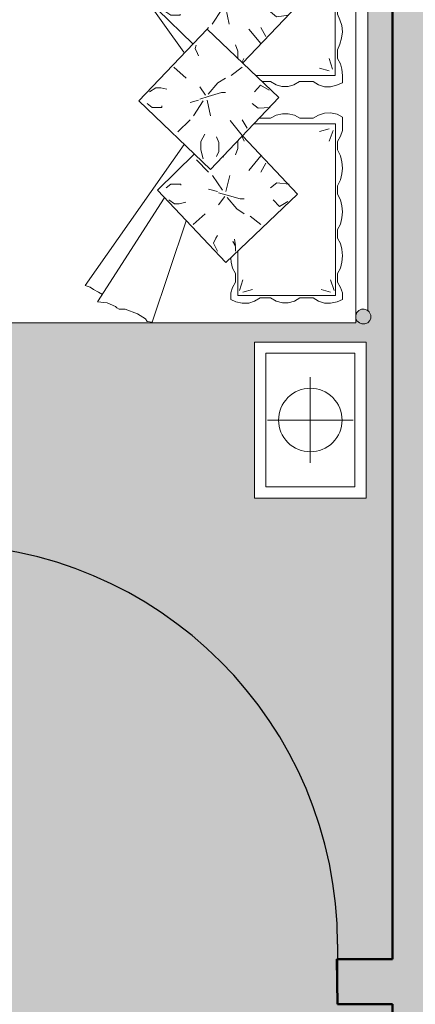
# Model space of a CAD drawing. Units: inches. Extents: x 528 to 2620, y -1066 to 798.
# Tile 11 of 41: x 737 to 776, y 573 to 672. Entities that reach past the tile are written whole.
import ezdxf

# ---------------------------------------------------------------- set-up
doc = ezdxf.new("R2010")
doc.units = ezdxf.units.IN
doc.header["$MEASUREMENT"] = 0
for name, color, linetype, lineweight in [('A-Door', 2, 'Continuous', 25), ('A-FURN', 30, 'Continuous', 18), ('A-WALL', 7, 'Continuous', 50), ('A-WALL-PATT', 8, 'Continuous', 13)]:
    doc.layers.add(name, color=color, linetype=linetype, lineweight=lineweight)

# ---------------------------------------------------------------- blocks, each defined once
blk = doc.blocks.new('*U4')
for p, q in [((0, 0), (0, -6)), ((40, 0), (40, -6))]:
    blk.add_line(p, q)
blk.add_lwpolyline([(0, 0), (0, 40), (1.75, 40), (1.75, 0)], close=True)
blk.add_arc((0, 0), 40, 0, 90)
blk = doc.blocks.new('d-bed-3')
at = {"color": 0, "linetype": 'ByBlock'}
for p, q in [((0, 0), (0, -0.5)), ((0.7, 0), (0, 0)), ((0.7, -0.5), (0.7, 0)), ((0.7817, -0.0054), (0.7857, 0.0078)), ((0.7817, -0.0054), (0.7857, 0.0078)), ((0.7857, 0.0078), (0.7968, 0.0166)), ((0.7857, 0.0078), (0.7968, 0.0166)), ((0.7968, 0.0166), (0.8078, 0.0211)), ((0.7968, 0.0166), (0.8078, 0.0211)), ((0.8078, 0.0211), (0.8209, 0.0211)), ((0.8078, 0.0211), (0.8209, 0.0211)), ((0.8209, 0.0211), (0.8349, 0.0144)), ((0.8209, 0.0211), (0.8349, 0.0144)), ((0.8349, 0.0144), (0.8409, 0.0078)), ((0.8349, 0.0144), (0.8429, 0.0056)), ((0.8389, 0.0078), (2.7305, 0.0078)), ((0.8409, 0.0078), (2.7305, 0.0078)), ((0.8429, 0.0056), (0.848, -0.0077)), ((2.7234, -0.0077), (2.7284, 0.0056)), ((2.7284, 0.0056), (2.7365, 0.0144)), ((2.7305, 0.0078), (2.7365, 0.0144)), ((2.7365, 0.0144), (2.7505, 0.0211)), ((2.7365, 0.0144), (2.7505, 0.0211)), ((2.7505, 0.0211), (2.7636, 0.0211)), ((2.7505, 0.0211), (2.7636, 0.0211)), ((2.7636, 0.0211), (2.7746, 0.0166)), ((2.7636, 0.0211), (2.7746, 0.0166)), ((2.7746, 0.0166), (2.7857, 0.0078)), ((2.7746, 0.0166), (2.7857, 0.0078)), ((2.7857, 0.0078), (2.7897, -0.0054)), ((2.7857, 0.0078), (2.7897, -0.0054)), ((2.8714, -0.5), (2.8714, 0)), ((2.8714, 0), (3.5714, 0)), ((3.5714, 0), (3.5714, -0.5)), ((0.7817, -0.0187), (0.7817, -0.0054)), ((0.7817, -0.0187), (0.7817, -0.0054)), ((0.7857, -0.0297), (0.7817, -0.0187)), ((0.7857, -0.0297), (0.7817, -0.0187)), ((0.7857, -2.0939), (0.7857, -0.0297)), ((0.7948, -0.0408), (0.7857, -0.0297)), ((0.7857, -0.032), (0.7857, -2.0939)), ((0.8058, -0.0452), (0.7948, -0.0408)), ((0.8319, -0.0408), (0.8188, -0.0452)), ((0.8409, -0.032), (0.8319, -0.0408)), ((0.848, -0.0209), (0.8409, -0.032)), ((0.848, -0.0077), (0.848, -0.0209)), ((2.7234, -0.0209), (2.7234, -0.0077)), ((2.7305, -0.032), (2.7234, -0.0209)), ((2.7395, -0.0408), (2.7305, -0.032)), ((2.7525, -0.0452), (2.7395, -0.0408)), ((2.7766, -0.0408), (2.7656, -0.0452)), ((2.7766, -0.0408), (2.7656, -0.0452)), ((2.7857, -0.0297), (2.7766, -0.0408)), ((2.7857, -0.0297), (2.7766, -0.0408)), ((2.7897, -0.0187), (2.7857, -0.0297)), ((2.7897, -0.0187), (2.7857, -0.0297)), ((2.7897, -0.0054), (2.7897, -0.0187)), ((2.7897, -0.0054), (2.7897, -0.0187)), ((0.05, -0.05), (0.05, -0.45)), ((0.65, -0.05), (0.05, -0.05)), ((0.35, -0.0576), (0.35, -0.4424)), ((0.65, -0.45), (0.65, -0.05)), ((0.8188, -0.0452), (0.8058, -0.0452)), ((2.7525, -0.0452), (0.8188, -0.0452)), ((2.7656, -0.0452), (2.7525, -0.0452)), ((2.7656, -0.0452), (2.7857, -0.0452)), ((2.7857, -0.0452), (2.7656, -0.0452)), ((2.7857, -2.0939), (2.7857, -0.0452)), ((2.9214, -0.45), (2.9214, -0.05)), ((2.9214, -0.05), (3.5214, -0.05)), ((3.2214, -0.0576), (3.2214, -0.4424)), ((3.5214, -0.05), (3.5214, -0.45)), ((0.8721, -0.159), (0.8781, -0.1325)), ((0.8781, -0.1325), (0.8911, -0.1059)), ((0.8911, -0.1059), (0.9182, -0.1082)), ((0.9182, -0.1082), (0.9443, -0.1148)), ((0.9443, -0.1148), (0.9684, -0.128)), ((0.9684, -0.128), (1.0056, -0.128)), ((1.0056, -0.128), (1.0317, -0.117)), ((1.0317, -0.117), (1.0588, -0.1082)), ((1.0588, -0.1082), (1.0849, -0.1059)), ((1.0849, -0.1059), (1.113, -0.1104)), ((1.113, -0.1104), (1.1401, -0.117)), ((1.1401, -0.117), (1.1662, -0.128)), ((1.1662, -0.128), (1.2034, -0.128)), ((1.2034, -0.128), (1.2295, -0.117)), ((1.2295, -0.117), (1.2566, -0.1082)), ((1.2566, -0.1082), (1.2827, -0.1059)), ((1.2827, -0.1059), (1.3108, -0.1104)), ((1.3108, -0.1104), (1.3379, -0.117)), ((1.3379, -0.117), (1.362, -0.128)), ((1.362, -0.128), (1.4012, -0.128)), ((1.4012, -0.128), (1.4253, -0.117)), ((1.4253, -0.117), (1.4514, -0.1082)), ((1.4514, -0.1082), (1.4805, -0.1059)), ((1.4805, -0.1059), (1.5086, -0.1104)), ((1.5086, -0.1104), (1.5357, -0.117)), ((1.5357, -0.117), (1.5598, -0.128)), ((1.5598, -0.128), (1.5989, -0.128)), ((1.5989, -0.128), (1.623, -0.1148)), ((1.623, -0.1148), (1.6471, -0.1082)), ((1.6471, -0.1082), (1.6763, -0.1059)), ((1.6763, -0.1059), (1.7084, -0.1059)), ((1.7084, -0.1059), (1.7194, -0.1325)), ((1.7194, -0.1325), (1.7265, -0.159)), ((1.8429, -0.159), (1.8489, -0.1302)), ((1.8489, -0.1302), (1.863, -0.1059)), ((1.863, -0.1059), (1.8951, -0.1059)), ((1.8951, -0.1059), (1.9222, -0.1059)), ((1.9222, -0.1059), (1.9483, -0.1148)), ((1.9483, -0.1148), (1.9724, -0.128)), ((1.9724, -0.128), (2.0096, -0.128)), ((2.0096, -0.128), (2.0357, -0.1148)), ((2.0357, -0.1148), (2.0628, -0.1082)), ((2.0628, -0.1082), (2.0909, -0.1059)), ((2.0909, -0.1059), (2.117, -0.1082)), ((2.117, -0.1082), (2.1441, -0.1148)), ((2.1441, -0.1148), (2.1702, -0.128)), ((2.1702, -0.128), (2.2074, -0.128)), ((2.2074, -0.128), (2.2335, -0.1148)), ((2.2335, -0.1148), (2.2606, -0.1082)), ((2.2606, -0.1082), (2.2867, -0.1059)), ((2.2867, -0.1059), (2.3148, -0.1082)), ((2.3148, -0.1082), (2.3419, -0.1148)), ((2.3419, -0.1148), (2.366, -0.128)), ((2.366, -0.128), (2.4052, -0.128)), ((2.4052, -0.128), (2.4293, -0.1148)), ((2.4293, -0.1148), (2.4554, -0.1082)), ((2.4554, -0.1082), (2.4845, -0.1059)), ((2.4845, -0.1059), (2.5126, -0.1082)), ((2.5126, -0.1082), (2.5397, -0.1148)), ((2.5397, -0.1148), (2.5638, -0.128)), ((2.5638, -0.128), (2.6029, -0.128)), ((2.6029, -0.128), (2.627, -0.1148)), ((2.627, -0.1148), (2.6511, -0.1059)), ((2.6511, -0.1059), (2.6803, -0.1059)), ((2.6803, -0.1059), (2.6913, -0.1302)), ((2.6913, -0.1302), (2.6973, -0.159)), ((0.8741, -0.1866), (0.8721, -0.159)), ((0.9072, -0.5753), (0.9072, -0.1391)), ((0.9072, -0.1391), (1.6763, -0.1391)), ((0.9223, -0.1612), (0.9333, -0.2042)), ((0.9293, -0.1435), (0.9775, -0.1612)), ((1.6471, -0.1501), (1.5989, -0.1656)), ((1.6542, -0.1656), (1.6431, -0.2087)), ((1.6763, -0.1391), (1.6763, -0.4936)), ((1.7265, -0.159), (1.7265, -0.1866)), ((1.8449, -0.1866), (1.8429, -0.159)), ((2.6622, -0.1369), (1.8931, -0.1369)), ((1.8931, -0.1369), (1.8931, -0.5046)), ((1.9152, -0.1656), (1.9263, -0.2087)), ((1.9222, -0.1479), (1.9704, -0.1656)), ((2.6401, -0.1435), (2.5919, -0.159)), ((2.6471, -0.159), (2.6361, -0.202)), ((2.6622, -0.5753), (2.6622, -0.1369)), ((2.6973, -0.159), (2.6973, -0.1866)), ((0.8831, -0.2131), (0.8741, -0.1866)), ((0.8962, -0.2374), (0.8831, -0.2131)), ((1.7174, -0.2131), (1.7024, -0.2374)), ((1.7265, -0.1866), (1.7174, -0.2131)), ((1.854, -0.2131), (1.8449, -0.1866)), ((1.867, -0.2374), (1.854, -0.2131)), ((2.6883, -0.2131), (2.6732, -0.2374)), ((2.6973, -0.1866), (2.6883, -0.2131)), ((0.1576, -0.25), (0.5424, -0.25)), ((0.8962, -0.2992), (0.8962, -0.2374)), ((1.7024, -0.2374), (1.7024, -0.2992)), ((1.867, -0.297), (1.867, -0.2374)), ((2.6732, -0.2374), (2.6732, -0.297)), ((3.4138, -0.25), (3.029, -0.25)), ((0.8831, -0.3235), (0.8962, -0.2992)), ((1.0538, -0.6294), (1.362, -0.3081)), ((1.362, -0.3081), (1.619, -0.5532)), ((1.7024, -0.2992), (1.7174, -0.3235)), ((1.854, -0.3213), (1.867, -0.297)), ((2.2074, -0.3081), (1.9483, -0.5532)), ((2.5146, -0.6294), (2.2074, -0.3081)), ((2.6732, -0.297), (2.6883, -0.3213)), ((0.8761, -0.3489), (0.8831, -0.3235)), ((0.8761, -0.3776), (0.8761, -0.3489)), ((1.3289, -0.3511), (1.3068, -0.3909)), ((1.4052, -0.3467), (1.4122, -0.4019)), ((1.7174, -0.3235), (1.7244, -0.3489)), ((1.7244, -0.3489), (1.7244, -0.3776)), ((1.8469, -0.3489), (1.854, -0.3213)), ((1.8469, -0.3754), (1.8469, -0.3489)), ((2.1632, -0.3445), (2.1572, -0.3997)), ((2.2405, -0.3511), (2.2626, -0.3887)), ((2.6883, -0.3213), (2.6953, -0.3489)), ((2.6953, -0.3489), (2.6953, -0.3754)), ((0.8831, -0.4041), (0.8761, -0.3776)), ((1.3068, -0.3909), (1.3349, -0.4174)), ((1.4674, -0.7134), (1.7746, -0.3909)), ((1.7244, -0.3776), (1.7174, -0.4041)), ((1.7746, -0.3909), (2.0979, -0.6979)), ((1.854, -0.4041), (1.8469, -0.3754)), ((2.2626, -0.3887), (2.2335, -0.4174)), ((2.6953, -0.3754), (2.6883, -0.4041)), ((0.8962, -0.4284), (0.8831, -0.4041)), ((0.8962, -0.4781), (0.8962, -0.4284)), ((1.4122, -0.4019), (1.3901, -0.4284)), ((1.7174, -0.4041), (1.7024, -0.4284)), ((1.7024, -0.4284), (1.7024, -0.4649)), ((1.7415, -0.4351), (1.7194, -0.4737)), ((1.8188, -0.4306), (1.8228, -0.4848)), ((1.867, -0.4284), (1.854, -0.4041)), ((1.867, -0.4781), (1.867, -0.4284)), ((2.1572, -0.3997), (2.1793, -0.4284)), ((2.6883, -0.4041), (2.6732, -0.4284)), ((2.6732, -0.4284), (2.6732, -0.4759)), ((0.05, -0.45), (0.65, -0.45)), ((0.8831, -0.5024), (0.8962, -0.4781)), ((1.2255, -0.4715), (1.2626, -0.5223)), ((1.5006, -0.4505), (1.4604, -0.4715)), ((1.5327, -0.4715), (1.4674, -0.5267)), ((1.7194, -0.4737), (1.7485, -0.5002)), ((1.8228, -0.4848), (1.8008, -0.5113)), ((2.0357, -0.4715), (2.102, -0.5267)), ((2.0688, -0.4505), (2.109, -0.4715)), ((2.3439, -0.4715), (2.3068, -0.5201)), ((2.6732, -0.4759), (2.6883, -0.5002)), ((3.5214, -0.45), (2.9214, -0.45)), ((0, -0.5), (0.7, -0.5)), ((0.8721, -0.5576), (0.8741, -0.5289)), ((0.8741, -0.5289), (0.8831, -0.5024)), ((0.9223, -0.5532), (0.9333, -0.5113)), ((2.6471, -0.5532), (2.6361, -0.5091)), ((2.6883, -0.5002), (2.6973, -0.5267)), ((2.6973, -0.5267), (2.6973, -0.5554)), ((3.5714, -0.5), (2.8714, -0.5)), ((0.8781, -0.5841), (0.8721, -0.5576)), ((0.9293, -0.5709), (0.9775, -0.5532)), ((1.2957, -0.5819), (1.2737, -0.5488)), ((1.3399, -0.5643), (1.3399, -0.5488)), ((1.357, -0.625), (1.3399, -0.5643)), ((1.5989, -0.5488), (1.614, -0.5554)), ((1.6381, -0.5554), (1.6763, -0.6051)), ((1.9112, -0.5333), (1.874, -0.5554)), ((1.9443, -0.5554), (1.8781, -0.6096)), ((1.9704, -0.5466), (1.9503, -0.5554)), ((2.2124, -0.6228), (2.2295, -0.5643)), ((2.2295, -0.5643), (2.2295, -0.5466)), ((2.2736, -0.5797), (2.2957, -0.5466)), ((2.6401, -0.5687), (2.5919, -0.5532)), ((2.6973, -0.5554), (2.6913, -0.5841)), ((0.8911, -0.6096), (0.8781, -0.5841)), ((0.9182, -0.6073), (0.8911, -0.6096)), ((1.109, -0.5753), (0.9072, -0.5753)), ((0.9443, -0.6007), (0.9182, -0.6073)), ((0.9684, -0.5886), (0.9443, -0.6007)), ((1.0056, -0.5886), (0.9684, -0.5886)), ((1.0317, -0.5996), (1.0056, -0.5886)), ((1.0588, -0.6073), (1.0317, -0.5996)), ((1.0759, -0.6096), (1.0588, -0.6073)), ((1.105, -0.5864), (1.1271, -0.5864)), ((1.1271, -0.5864), (1.1482, -0.5974)), ((1.1482, -0.5974), (1.1311, -0.5864)), ((1.1311, -0.5864), (1.1592, -0.593)), ((1.3459, -0.625), (1.2957, -0.5819)), ((1.3731, -0.6294), (1.4453, -0.614)), ((1.5658, -0.5753), (1.5377, -0.5864)), ((1.5969, -0.5753), (1.5658, -0.5753)), ((1.9684, -0.5753), (2.0036, -0.5753)), ((2.0036, -0.5753), (2.0317, -0.5864)), ((2.1963, -0.6294), (2.124, -0.6118)), ((2.2224, -0.6228), (2.2736, -0.5797)), ((2.4383, -0.5864), (2.4092, -0.5908)), ((2.4423, -0.5864), (2.4202, -0.5974)), ((2.4202, -0.5974), (2.4383, -0.5864)), ((2.4644, -0.5864), (2.4423, -0.5864)), ((2.4604, -0.5753), (2.6622, -0.5753)), ((2.5126, -0.6051), (2.4955, -0.6073)), ((2.5397, -0.5996), (2.5126, -0.6051)), ((2.5638, -0.5864), (2.5397, -0.5996)), ((2.6029, -0.5864), (2.5638, -0.5864)), ((2.627, -0.5996), (2.6029, -0.5864)), ((2.6511, -0.6073), (2.627, -0.5996)), ((2.6803, -0.6073), (2.6511, -0.6073)), ((2.6913, -0.5841), (2.6803, -0.6073)), ((1.3791, -0.9365), (1.0538, -0.6294)), ((1.3138, -0.6626), (1.351, -0.6361)), ((1.368, -0.6626), (1.357, -0.625)), ((1.3791, -0.6471), (1.4453, -0.6913)), ((1.7084, -0.6648), (1.6873, -0.6316)), ((1.7526, -0.6493), (1.7526, -0.6316)), ((1.7706, -0.7089), (1.7526, -0.6493)), ((1.9765, -0.6604), (1.9503, -0.6714)), ((2.0166, -0.6604), (1.9765, -0.6604)), ((2.0387, -0.6714), (2.0166, -0.6604)), ((2.0387, -0.6427), (2.0427, -0.6405)), ((2.1903, -0.6449), (2.124, -0.6891)), ((2.1903, -0.9365), (2.5146, -0.6294)), ((2.2013, -0.6626), (2.2124, -0.6228)), ((2.2556, -0.6626), (2.2184, -0.6338)), ((1.105, -0.6692), (1.1421, -0.6846)), ((1.1421, -0.6846), (1.1642, -0.6736)), ((1.1642, -0.6736), (1.1753, -0.6692)), ((1.3731, -0.6692), (1.3841, -0.7067)), ((1.7596, -0.7089), (1.7084, -0.6648)), ((1.7857, -0.7134), (1.856, -0.6979)), ((2.0979, -0.6979), (1.7897, -1.0193)), ((2.1963, -0.667), (2.1853, -0.7067)), ((2.4052, -0.6736), (2.3941, -0.667)), ((2.4272, -0.6846), (2.4052, -0.6736)), ((2.4644, -0.667), (2.4272, -0.6846)), ((1.2255, -0.7785), (1.2737, -0.7244)), ((1.4674, -0.7134), (1.4604, -0.7067)), ((1.7897, -1.0193), (1.4674, -0.7134)), ((1.7265, -0.7454), (1.7636, -0.72)), ((1.7817, -0.7454), (1.7706, -0.7089)), ((1.7897, -0.731), (1.856, -0.7741)), ((1.9724, -0.741), (1.9393, -0.7244)), ((2.0096, -0.741), (1.9724, -0.741)), ((2.0497, -0.731), (2.0096, -0.741)), ((2.0538, -0.7609), (2.109, -0.7067)), ((2.3439, -0.7763), (2.2957, -0.7222)), ((1.3791, -0.9365), (1.5357, -0.7763)), ((1.5548, -0.7675), (1.5397, -0.7631)), ((1.5548, -0.7675), (1.5769, -0.7564)), ((1.5769, -0.7564), (1.5879, -0.752)), ((1.7857, -0.752), (1.7967, -0.7896)), ((1.9283, -0.8448), (1.874, -0.7896)), ((2.1903, -0.9365), (2.0277, -0.7697)), ((0.7857, -0.9607), (1.2295, -0.8072)), ((0.9504, -1.2611), (1.5708, -0.8183)), ((1.3178, -0.8382), (1.3239, -0.8117)), ((1.3178, -0.8602), (1.3178, -0.8382)), ((1.4052, -0.8337), (1.4012, -0.8337)), ((1.4052, -0.8768), (1.4052, -0.8337)), ((1.6381, -0.8625), (1.6873, -0.8072)), ((2.618, -1.2611), (1.9855, -0.8161)), ((2.1632, -0.8757), (2.1632, -0.8315)), ((2.1632, -0.8315), (2.1682, -0.8315)), ((2.2515, -0.8382), (2.2445, -0.8094)), ((2.2515, -0.8602), (2.2515, -0.8382)), ((2.7827, -0.9607), (2.3278, -0.8072)), ((1.3349, -0.8879), (1.3178, -0.8602)), ((1.3901, -0.8989), (1.4052, -0.8768)), ((2.1793, -0.8967), (2.1632, -0.8757)), ((2.2335, -0.8856), (2.2515, -0.8602)), ((0.8781, -1.2059), (1.3349, -0.9055)), ((1.7305, -0.921), (1.7375, -0.8945)), ((1.7305, -0.9431), (1.7305, -0.921)), ((1.8188, -0.9166), (1.8118, -0.9166)), ((1.8188, -0.9607), (1.8188, -0.9166)), ((2.6913, -1.2059), (2.2254, -0.9055)), ((0.8128, -1.0115), (0.7857, -0.9607)), ((1.7485, -0.9718), (1.7305, -0.9431)), ((1.8008, -0.9828), (1.8188, -0.9607)), ((2.7827, -0.9607), (2.7786, -0.9828)), ((0.8128, -1.0325), (0.8128, -1.0115)), ((2.7676, -0.9895), (2.7455, -1.0259)), ((2.7786, -0.9828), (2.7676, -0.9895)), ((0.8239, -1.0414), (0.8128, -1.0325)), ((0.8299, -1.0635), (0.8239, -1.0414)), ((2.7455, -1.0259), (2.7234, -1.0811)), ((0.8349, -1.0745), (0.8299, -1.0635)), ((0.845, -1.1032), (0.8349, -1.0745)), ((0.852, -1.1187), (0.845, -1.1032)), ((2.7234, -1.0811), (2.7234, -1.1076)), ((0.852, -1.1363), (0.852, -1.1187)), ((0.863, -1.1617), (0.852, -1.1363)), ((2.7124, -1.1253), (2.6953, -1.1617)), ((2.7174, -1.1187), (2.7124, -1.1253)), ((2.7234, -1.1076), (2.7174, -1.1187)), ((0.867, -1.1905), (0.863, -1.1617)), ((0.8741, -1.1949), (0.867, -1.1905)), ((0.9223, -1.2015), (0.9112, -1.1838)), ((2.6582, -1.1838), (2.6471, -1.2015)), ((2.6953, -1.1617), (2.6913, -1.2059)), ((0.8781, -1.2059), (0.8741, -1.1949)), ((0.9293, -1.2059), (0.9223, -1.2015)), ((0.9403, -1.2236), (0.9293, -1.2059)), ((0.9443, -1.2391), (0.9403, -1.2236)), ((2.6361, -1.2236), (2.625, -1.2391)), ((2.6471, -1.2015), (2.6361, -1.2236)), ((0.9504, -1.2611), (0.9443, -1.2391)), ((2.625, -1.2391), (2.618, -1.2611)), ((0.8741, -2.0673), (0.9464, -1.9691)), ((2.7234, -2.0497), (2.6913, -1.947)), ((0.8851, -2.1005), (0.9795, -2.0342)), ((2.7305, -2.0939), (2.6421, -2.0342)), ((0.7888, -2.1317), (0.7857, -2.0939)), ((0.7857, -2.0939), (0.7887, -2.1303)), ((2.7857, -2.0939), (2.7783, -2.1299)), ((2.7786, -2.1281), (2.7857, -2.0939)), ((0.7797, -2.148), (0.7857, -2.1347)), ((0.7797, -2.148), (0.7857, -2.1347)), ((0.7797, -2.159), (0.7797, -2.148)), ((0.7797, -2.148), (0.7797, -2.159)), ((0.7837, -2.1723), (0.7797, -2.159)), ((0.7837, -2.1723), (0.7797, -2.159)), ((0.7857, -2.1347), (0.7948, -2.1259)), ((0.7857, -2.1347), (0.7888, -2.1317)), ((0.7948, -2.1259), (0.8078, -2.1215)), ((0.8078, -2.1215), (0.8188, -2.1215)), ((0.8188, -2.1215), (0.8319, -2.1281)), ((0.8319, -2.1281), (0.8409, -2.1369)), ((0.845, -2.1612), (0.8389, -2.1745)), ((0.8409, -2.1369), (0.845, -2.1502)), ((2.7264, -2.1436), (0.845, -2.1436)), ((0.845, -2.1502), (0.845, -2.1612)), ((2.7284, -2.1369), (2.7234, -2.1502)), ((2.7234, -2.1502), (2.7234, -2.1612)), ((2.7234, -2.1612), (2.7305, -2.1745)), ((2.7365, -2.1281), (2.7284, -2.1369)), ((2.7505, -2.1215), (2.7365, -2.1281)), ((2.7616, -2.1215), (2.7505, -2.1215)), ((2.7746, -2.1259), (2.7616, -2.1215)), ((2.7827, -2.1347), (2.7746, -2.1259)), ((2.7783, -2.1299), (2.7827, -2.1347)), ((2.7827, -2.1347), (2.7897, -2.148)), ((2.7897, -2.148), (2.7827, -2.1347)), ((2.7897, -2.159), (2.7857, -2.1723)), ((2.7857, -2.1723), (2.7897, -2.159)), ((2.7897, -2.148), (2.7897, -2.159)), ((2.7897, -2.159), (2.7897, -2.148)), ((0.7927, -2.1811), (0.7837, -2.1723)), ((0.7927, -2.1811), (0.7837, -2.1723)), ((0.8058, -2.1877), (0.7927, -2.1811)), ((0.8058, -2.1877), (0.7927, -2.1811)), ((0.8168, -2.1877), (0.8058, -2.1877)), ((0.8168, -2.1877), (0.8058, -2.1877)), ((0.8299, -2.1833), (0.8168, -2.1877)), ((0.8299, -2.1833), (0.8168, -2.1877)), ((0.8389, -2.1745), (0.8299, -2.1833)), ((0.8367, -2.1767), (0.8299, -2.1833)), ((2.7327, -2.1767), (0.8367, -2.1767)), ((0.8389, -2.1767), (2.7305, -2.1767)), ((2.7305, -2.1745), (2.7395, -2.1833)), ((2.7395, -2.1833), (2.7327, -2.1767)), ((2.7525, -2.1877), (2.7395, -2.1833)), ((2.7395, -2.1833), (2.7525, -2.1877)), ((2.7636, -2.1877), (2.7525, -2.1877)), ((2.7525, -2.1877), (2.7636, -2.1877)), ((2.7766, -2.1811), (2.7636, -2.1877)), ((2.7636, -2.1877), (2.7766, -2.1811)), ((2.7857, -2.1723), (2.7766, -2.1811)), ((2.7766, -2.1811), (2.7857, -2.1723))]:
    blk.add_line(p, q, dxfattribs=at)
blk.add_ellipse((0.35, -0.25), major_axis=(-0.1007, 0.1007), ratio=1, dxfattribs=at)
at = {"color": 0, "linetype": 'ByBlock', "extrusion": (0, 0, -1)}
blk.add_ellipse((3.2214, -0.25), major_axis=(0.1007, 0.1007), ratio=1, dxfattribs=at)

msp = doc.modelspace()

# ---------------------------------------------------------------- hatches: boundary and pattern name
at = {"layer": 'A-WALL-PATT', "transparency": 33554521}
h = msp.add_hatch(color=256, dxfattribs=at)
h.dxf.hatch_style = 1
h.paths.add_polyline_path([(629.059, 709.922), (677.559, 709.922), (677.559, 718.922), (620.059, 718.922), (620.059, 667.922), (629.059, 667.922)])
h.paths.add_polyline_path([(790.559, 718.922), (725.559, 718.922), (725.559, 709.922), (774.059, 709.922), (774.059, 577.922), (768.481, 577.922), (768.559, 573.422), (774.059, 573.422), (774.059, 567.422), (778.559, 567.422), (778.559, 669.422), (831.059, 669.422), (831.059, 675.922), (826.559, 675.922), (826.559, 673.922), (778.559, 673.922), (778.559, 709.922), (790.559, 709.922)])
h.paths.add_polyline_path([(908.059, 718.922), (879.059, 718.922), (879.059, 709.922), (899.059, 709.922), (899.059, 641.672), (908.059, 641.672)])
h.paths.add_polyline_path([(629.059, 619.922), (620.059, 619.922), (620.059, 561.422), (629.059, 561.422), (629.059, 573.422), (724.059, 573.422), (724.059, 569.422), (728.559, 569.422), (728.559, 577.922), (629.059, 577.922)])
h.paths.add_polyline_path([(779.059, 391.422), (779.059, 400.422), (770.059, 400.422), (764.059, 400.422), (764.059, 397.422), (764.059, 391.422), (770.059, 391.422), (770.059, 268.922), (815.059, 268.922), (815.059, 277.922), (779.059, 277.922), (779.059, 359.767)])
h.paths.add_polyline_path([(908.059, 395.922), (899.059, 395.922), (851.059, 395.922), (851.059, 391.422), (899.059, 391.422), (899.059, 277.922), (863.059, 277.922), (863.059, 268.922), (908.059, 268.922)])
h.paths.add_polyline_path([(908.059, 593.672), (899.059, 593.672), (899.059, 525.422), (778.559, 525.422), (778.559, 527.172), (774.059, 527.172), (774.059, 520.922), (899.059, 520.922), (899.059, 443.922), (908.059, 443.922)])
h.paths.add_polyline_path([(629.059, 520.922), (728.559, 520.922), (728.559, 545.422), (724.059, 545.422), (724.059, 525.422), (629.059, 525.422), (629.059, 537.422), (620.059, 537.422), (620.059, 484.672), (629.059, 484.672)])
h.paths.add_polyline_path([(629.059, 436.672), (620.059, 436.672), (620.059, 391.422), (648.559, 391.422), (648.559, 400.422), (629.059, 400.422)])
h.paths.add_polyline_path([(716.059, 397.422), (716.059, 400.422), (696.559, 400.422), (696.559, 391.422), (716.059, 391.422)])
at = {"layer": 'A-WALL-PATT', "transparency": 33554590}
h = msp.add_hatch(color=256, dxfattribs=at)
h.dxf.hatch_style = 1
h.paths.add_polyline_path([(774.059, 709.922), (629.059, 709.922), (629.059, 577.922), (728.559, 577.922), (728.559, 579.422), (728.559, 619.422), (730.309, 619.422), (730.309, 619.384, -0.401453), (768.559, 579.422), (768.559, 577.922), (774.059, 577.922)])
h.paths.add_polyline_path([(723.896, 686.058), (723.968, 686.064), (723.828, 686.128)], flags=0)
h.paths.add_polyline_path([(722.785, 642.699), (722.893, 642.756), (722.893, 684.992), (722.647, 685.244), (722.647, 685.82), (723.079, 686.262), (723.533, 686.262), (723.968, 686.064), (724.739, 686.128), (770.696, 686.128), (770.78, 686.14), (771.126, 686.266), (771.694, 686.094), (771.94, 685.478), (771.67, 684.904), (771.582, 684.871), (771.582, 642.782), (771.878, 642.514), (771.878, 641.921), (771.511, 641.462), (770.855, 641.462), (770.401, 641.833), (770.401, 641.551), (724.739, 641.551), (723.991, 641.705), (723.443, 641.414), (722.879, 641.585), (722.597, 642.142)], flags=16)
h.paths.add_polyline_path([(723.994, 641.704), (723.994, 641.707), (723.991, 641.705)], flags=0)
h.paths.add_polyline_path([(722.893, 642.732), (722.893, 684.992), (722.647, 685.244), (722.647, 685.82), (723.079, 686.262), (723.287, 686.262), (722.991, 686.172), (722.794, 685.971), (722.647, 685.68), (722.647, 685.434), (722.745, 685.143), (722.942, 684.942), (723.238, 684.807), (723.484, 684.807), (723.779, 684.897), (723.976, 685.098), (724.174, 685.488), (724.124, 685.635), (724.124, 685.249), (723.631, 684.746), (723.631, 642.961), (724.124, 642.514), (724.124, 641.887), (723.656, 641.462), (723.079, 641.462), (722.647, 641.904), (722.647, 642.48)], flags=0)
h.paths.add_polyline_path([(722.647, 642.29), (722.647, 642.044), (722.794, 641.753), (723.079, 641.462), (723.287, 641.462), (722.879, 641.585), (722.597, 642.142)], flags=0)
h.paths.add_polyline_path([(770.745, 686.128), (770.58, 686.128), (770.551, 686.057)], flags=0)
h.paths.add_polyline_path([(743.299, 645.288), (753.227, 659.398), (748.69, 663.75), (753.234, 668.538), (743.299, 682.458), (743.791, 682.592), (744.136, 682.681), (744.53, 682.928), (744.628, 683.084), (745.017, 683.327), (744.53, 684.069), (744.776, 684.158), (744.874, 684.315), (745.514, 684.404), (746.081, 684.651), (746.474, 684.651), (746.819, 684.807), (747.459, 685.031), (747.705, 685.143), (748.198, 685.277), (748.394, 685.523), (748.862, 685.523), (749.994, 686.128), (753.488, 676.03), (757.379, 680.153), (757.791, 679.758), (758.044, 680.645), (758.29, 681.227), (758.29, 682.055), (758.019, 682.592), (757.871, 683.174), (757.822, 683.778), (758.388, 684.069), (758.979, 684.203), (759.619, 684.158), (760.21, 683.957), (760.751, 683.666), (761.859, 683.666), (762.401, 683.957), (762.991, 684.114), (763.631, 684.114), (764.198, 683.957), (764.739, 683.666), (766.118, 683.666), (766.659, 683.957), (767.25, 684.158), (767.865, 684.203), (768.456, 684.069), (769.047, 683.778), (768.998, 683.174), (768.85, 682.592), (768.554, 682.055), (768.554, 681.227), (768.801, 680.645), (769.092, 679.75), (768.948, 678.832), (768.801, 678.228), (768.554, 677.646), (768.554, 676.818), (768.801, 676.237), (769.092, 675.341), (768.948, 674.424), (768.801, 673.82), (768.554, 673.283), (768.554, 672.41), (768.801, 671.873), (768.998, 671.291), (769.047, 670.642), (768.948, 670.016), (768.801, 669.411), (768.554, 668.874), (768.554, 668.002), (768.974, 667.239), (769.047, 666.279), (769.047, 665.563), (768.456, 665.316), (767.865, 665.16), (767.25, 665.16), (766.659, 665.361), (766.118, 665.697), (764.739, 665.697), (763.945, 665.204), (762.991, 665.204), (762.401, 665.361), (761.859, 665.697), (761.005, 665.697), (762.696, 664.086), (760.741, 662.027), (761.859, 662.027), (762.401, 662.318), (763.342, 662.548), (764.247, 662.318), (764.788, 662.027), (766.118, 662.027), (766.659, 662.318), (767.25, 662.519), (767.865, 662.564), (768.505, 662.43), (769.047, 662.116), (769.047, 661.4), (769.047, 660.796), (768.85, 660.214), (768.554, 659.677), (768.554, 658.849), (768.85, 658.267), (768.998, 657.663), (769.069, 656.749), (768.85, 655.851), (768.554, 655.269), (768.554, 654.441), (768.85, 653.859), (769.069, 652.961), (768.998, 652.046), (768.85, 651.442), (768.554, 650.905), (768.554, 650.032), (768.85, 649.495), (768.998, 648.914), (769.047, 648.265), (768.998, 647.638), (768.85, 647.034), (768.554, 646.497), (768.554, 645.624), (768.85, 645.087), (769.047, 644.55), (769.047, 643.901), (768.505, 643.655), (767.865, 643.521), (767.25, 643.521), (766.659, 643.722), (766.118, 644.058), (764.788, 644.058), (764.247, 643.722), (763.342, 643.492), (762.401, 643.722), (761.859, 644.058), (760.801, 644.058), (760.259, 643.722), (759.668, 643.521), (759.028, 643.521), (758.388, 643.655), (757.871, 643.901), (757.871, 644.55), (758.044, 645.087), (758.339, 645.624), (758.339, 646.497), (758.044, 647.034), (757.921, 647.638), (757.866, 648.059), (757.379, 647.593), (753.422, 651.773), (749.994, 641.618), (749.502, 641.708), (749.354, 641.954), (748.542, 642.446), (747.311, 642.939), (746.652, 642.939), (746.327, 643.185), (745.514, 643.565), (744.53, 643.655), (745.011, 644.4), (744.628, 644.639), (744.136, 644.886), (743.791, 645.132)], flags=0)
h.paths.add_polyline_path([(755.656, 654.933), (756.542, 654.687), (757.527, 654.329), (756.641, 654.575)], flags=0)
h.paths.add_polyline_path([(758.339, 649.204), (758.339, 648.712), (758.585, 644.304), (758.585, 648.802)], flags=0)
h.paths.add_polyline_path([(758.339, 649.294), (758.093, 649.697), (758.359, 649.165)], flags=0)
h.paths.add_polyline_path([(755.656, 672.79), (756.493, 673.037), (757.358, 673.351), (757.353, 673.358), (756.641, 673.149)], flags=0)
h.paths.add_polyline_path([(760.264, 639.641), (771.408, 639.641), (771.408, 624.039), (760.264, 624.039)], flags=16)
h.paths.add_polyline_path([(761.378, 638.526), (770.294, 638.526), (770.294, 625.153), (761.378, 625.153)], flags=0)
edge = h.paths.add_edge_path(flags=0)
edge.add_ellipse((765.836, 631.84), major_axis=(-2.245, 2.245), ratio=1, start_angle=-45, end_angle=45, ccw=False)
edge.add_ellipse((765.836, 631.84), major_axis=(-2.245, 2.245), ratio=1, start_angle=-135, end_angle=-45, ccw=False)
edge.add_ellipse((765.836, 631.84), major_axis=(-2.245, 2.245), ratio=1, start_angle=135, end_angle=-135, ccw=False)
edge.add_ellipse((765.836, 631.84), major_axis=(-2.245, 2.245), ratio=1, start_angle=45, end_angle=135, ccw=False)
h.paths.add_polyline_path([(758.585, 683.42), (758.585, 678.922), (758.373, 678.575), (758.339, 678.43), (758.093, 678.049), (758.339, 678.519), (758.339, 679.011)], flags=0)
h.paths.add_polyline_path([(760.264, 688.038), (760.264, 703.64), (771.408, 703.64), (771.408, 688.038)], flags=16)
h.paths.add_polyline_path([(770.401, 685.389), (770.401, 685.846), (770.855, 686.217), (771.511, 686.217), (771.878, 685.758), (771.878, 685.165), (771.582, 684.897), (771.582, 642.782), (771.878, 642.514), (771.878, 641.921), (771.511, 641.462), (770.855, 641.462), (770.401, 641.833), (770.401, 642.29)], flags=0)
h.paths.add_polyline_path([(770.532, 642.678), (771.052, 643.009), (771.67, 642.775), (771.94, 642.201), (771.694, 641.585), (771.126, 641.413), (770.551, 641.622), (770.347, 642.132)], flags=16)
h.paths.add_polyline_path([(761.378, 689.152), (761.378, 702.526), (770.294, 702.526), (770.294, 689.152)], flags=0)
edge = h.paths.add_edge_path(flags=0)
edge.add_ellipse((765.836, 695.839), major_axis=(2.245, 2.245), ratio=1, start_angle=405, end_angle=495, ccw=False)
edge.add_ellipse((765.836, 695.839), major_axis=(2.245, 2.245), ratio=1, start_angle=675, end_angle=765, ccw=False)
edge.add_ellipse((765.836, 695.839), major_axis=(2.245, 2.245), ratio=1, start_angle=585, end_angle=675, ccw=False)
edge.add_ellipse((765.836, 695.839), major_axis=(2.245, 2.245), ratio=1, start_angle=495, end_angle=585, ccw=False)
h.paths.add_polyline_path([(770.696, 684.897), (770.942, 684.74), (771.41, 684.74), (771.73, 685.031), (771.878, 685.344), (771.878, 685.635), (771.694, 686.094), (771.582, 686.128), (771.878, 685.758), (771.878, 685.165), (771.41, 684.74), (770.849, 684.74)], flags=0)
h.paths.add_polyline_path([(899.059, 709.922), (831.059, 709.922), (831.059, 699.922), (829.809, 699.922), (829.809, 675.922), (831.059, 675.922), (831.059, 669.422), (778.559, 669.422), (778.559, 567.172), (780.059, 567.172), (820.059, 567.172), (820.059, 565.422), (820.021, 565.422, -0.401453), (780.059, 527.172), (778.559, 527.172), (778.559, 525.422), (899.059, 525.422)])
h.paths.add_polyline_path([(849.197, 636.014), (849.269, 636.02), (849.129, 636.084)], flags=0)
h.paths.add_polyline_path([(848.193, 634.948), (847.947, 635.2), (847.947, 635.776), (848.379, 636.218), (848.833, 636.218), (849.269, 636.02), (850.039, 636.084), (895.996, 636.084), (896.081, 636.096), (896.426, 636.222), (896.995, 636.05), (897.241, 635.434), (896.97, 634.86), (896.883, 634.827), (896.883, 592.738), (897.178, 592.47), (897.178, 591.877), (896.811, 591.418), (896.155, 591.418), (895.701, 591.789), (895.701, 591.507), (850.039, 591.507), (849.292, 591.661), (848.744, 591.37), (848.18, 591.541), (847.897, 592.098), (848.086, 592.655), (848.193, 592.712)], flags=16)
h.paths.add_polyline_path([(849.294, 591.66), (849.295, 591.663), (849.292, 591.661)], flags=16)
h.paths.add_polyline_path([(848.193, 634.948), (847.947, 635.2), (847.947, 635.776), (848.379, 636.218), (848.587, 636.218), (848.292, 636.128), (848.095, 635.927), (847.947, 635.636), (847.947, 635.39), (848.046, 635.099), (848.243, 634.897), (848.538, 634.763), (848.784, 634.763), (849.079, 634.853), (849.276, 635.054), (849.474, 635.444), (849.424, 635.591), (849.424, 635.205), (848.932, 634.702), (848.932, 592.917), (849.424, 592.47), (849.424, 591.843), (848.956, 591.418), (848.379, 591.418), (847.947, 591.86), (847.947, 592.436), (848.193, 592.688)], flags=0)
h.paths.add_polyline_path([(847.947, 592.246), (847.947, 592), (848.095, 591.709), (848.379, 591.418), (848.587, 591.418), (848.18, 591.541), (847.897, 592.098)], flags=16)
h.paths.add_polyline_path([(896.046, 636.084), (895.88, 636.084), (895.852, 636.013)], flags=0)
h.paths.add_polyline_path([(868.599, 632.414), (869.092, 632.548), (869.436, 632.637), (869.83, 632.884), (869.929, 633.04), (870.318, 633.283), (869.83, 634.025), (870.076, 634.114), (870.175, 634.271), (870.815, 634.36), (871.381, 634.607), (871.775, 634.607), (872.119, 634.763), (872.759, 634.987), (873.006, 635.099), (873.498, 635.233), (873.695, 635.479), (874.163, 635.479), (875.295, 636.084), (878.788, 625.986), (882.679, 630.109), (883.091, 629.714), (883.344, 630.601), (883.59, 631.183), (883.59, 632.011), (883.319, 632.548), (883.172, 633.13), (883.123, 633.734), (883.689, 634.025), (884.279, 634.159), (884.919, 634.114), (885.51, 633.913), (886.052, 633.622), (887.159, 633.622), (887.701, 633.913), (888.292, 634.07), (888.932, 634.07), (889.498, 633.913), (890.039, 633.622), (891.418, 633.622), (891.959, 633.913), (892.55, 634.114), (893.166, 634.159), (893.756, 634.025), (894.347, 633.734), (894.298, 633.13), (894.15, 632.548), (893.855, 632.011), (893.855, 631.183), (894.101, 630.601), (894.393, 629.706), (894.249, 628.788), (894.101, 628.184), (893.855, 627.602), (893.855, 626.774), (894.101, 626.193), (894.393, 625.297), (894.249, 624.38), (894.101, 623.776), (893.855, 623.239), (893.855, 622.366), (894.101, 621.829), (894.298, 621.247), (894.347, 620.598), (894.249, 619.972), (894.101, 619.367), (893.855, 618.83), (893.855, 617.958), (894.274, 617.195), (894.347, 616.235), (894.347, 615.518), (893.756, 615.272), (893.166, 615.116), (892.55, 615.116), (891.959, 615.317), (891.418, 615.653), (890.039, 615.653), (889.245, 615.16), (888.292, 615.16), (887.701, 615.317), (887.159, 615.653), (886.305, 615.653), (887.996, 614.042), (886.041, 611.983), (887.159, 611.983), (887.701, 612.274), (888.642, 612.504), (889.547, 612.274), (890.089, 611.983), (891.418, 611.983), (891.959, 612.274), (892.55, 612.475), (893.166, 612.52), (893.806, 612.386), (894.347, 612.072), (894.347, 611.356), (894.347, 610.752), (894.15, 610.17), (893.855, 609.633), (893.855, 608.805), (894.15, 608.223), (894.298, 607.619), (894.37, 606.705), (894.15, 605.807), (893.855, 605.225), (893.855, 604.397), (894.15, 603.815), (894.37, 602.917), (894.298, 602.002), (894.15, 601.398), (893.855, 600.861), (893.855, 599.988), (894.15, 599.451), (894.298, 598.87), (894.347, 598.221), (894.298, 597.594), (894.15, 596.99), (893.855, 596.453), (893.855, 595.58), (894.15, 595.043), (894.347, 594.506), (894.347, 593.857), (893.806, 593.611), (893.166, 593.477), (892.55, 593.477), (891.959, 593.678), (891.418, 594.014), (890.089, 594.014), (889.547, 593.678), (888.642, 593.448), (887.701, 593.678), (887.159, 594.014), (886.101, 594.014), (885.559, 593.678), (884.969, 593.477), (884.329, 593.477), (883.689, 593.611), (883.172, 593.857), (883.172, 594.506), (883.344, 595.043), (883.639, 595.58), (883.639, 596.453), (883.344, 596.99), (883.221, 597.594), (883.167, 598.015), (882.679, 597.549), (878.722, 601.729), (875.295, 591.574), (874.803, 591.664), (874.655, 591.91), (873.843, 592.402), (872.612, 592.895), (871.952, 592.895), (871.627, 593.141), (870.815, 593.521), (869.83, 593.611), (870.311, 594.356), (869.929, 594.595), (869.436, 594.842), (869.092, 595.088), (868.599, 595.244), (878.528, 609.354), (873.99, 613.706), (878.535, 618.494)], flags=0)
h.paths.add_polyline_path([(880.956, 622.746), (881.793, 622.993), (882.659, 623.307), (882.654, 623.314), (881.941, 623.104)], flags=0)
h.paths.add_polyline_path([(880.956, 604.889), (881.843, 604.643), (882.827, 604.285), (881.941, 604.531)], flags=16)
h.paths.add_polyline_path([(883.393, 628.005), (883.639, 628.475), (883.639, 628.967), (883.886, 633.376), (883.886, 628.878), (883.674, 628.531), (883.639, 628.386)], flags=0)
h.paths.add_polyline_path([(883.639, 599.16), (883.639, 598.668), (883.886, 594.26), (883.886, 598.758)], flags=16)
h.paths.add_polyline_path([(883.639, 599.25), (883.393, 599.653), (883.659, 599.121)], flags=16)
h.paths.add_polyline_path([(885.564, 637.994), (885.564, 653.596), (896.709, 653.596), (896.709, 637.994)], flags=16)
h.paths.add_polyline_path([(885.564, 589.597), (896.709, 589.597), (896.709, 573.995), (885.564, 573.995)], flags=16)
h.paths.add_polyline_path([(886.679, 639.108), (886.679, 652.482), (895.594, 652.482), (895.594, 639.108)], flags=0)
h.paths.add_polyline_path([(886.679, 588.482), (895.594, 588.482), (895.594, 575.109), (886.679, 575.109)], flags=0)
edge = h.paths.add_edge_path(flags=0)
edge.add_ellipse((891.136, 645.795), major_axis=(2.245, 2.245), ratio=1, start_angle=405, end_angle=495, ccw=False)
edge.add_ellipse((891.136, 645.795), major_axis=(2.245, 2.245), ratio=1, start_angle=675, end_angle=765, ccw=False)
edge.add_ellipse((891.136, 645.795), major_axis=(2.245, 2.245), ratio=1, start_angle=585, end_angle=675, ccw=False)
edge.add_ellipse((891.136, 645.795), major_axis=(2.245, 2.245), ratio=1, start_angle=495, end_angle=585, ccw=False)
edge = h.paths.add_edge_path(flags=0)
edge.add_ellipse((891.136, 581.796), major_axis=(-2.245, 2.245), ratio=1, start_angle=-45, end_angle=45, ccw=False)
edge.add_ellipse((891.136, 581.796), major_axis=(-2.245, 2.245), ratio=1, start_angle=-135, end_angle=-45, ccw=False)
edge.add_ellipse((891.136, 581.796), major_axis=(-2.245, 2.245), ratio=1, start_angle=135, end_angle=-135, ccw=False)
edge.add_ellipse((891.136, 581.796), major_axis=(-2.245, 2.245), ratio=1, start_angle=45, end_angle=135, ccw=False)
h.paths.add_polyline_path([(895.701, 635.345), (895.701, 635.802), (896.155, 636.173), (896.811, 636.173), (897.178, 635.714), (897.178, 635.121), (896.883, 634.853), (896.883, 592.738), (897.178, 592.47), (897.178, 591.877), (896.811, 591.418), (896.155, 591.418), (895.701, 591.789), (895.701, 592.246)], flags=0)
h.paths.add_polyline_path([(895.996, 634.853), (896.243, 634.696), (896.71, 634.696), (897.03, 634.987), (897.178, 635.3), (897.178, 635.591), (896.995, 636.05), (896.883, 636.084), (897.178, 635.714), (897.178, 635.121), (896.71, 634.696), (896.15, 634.696)], flags=0)
h.paths.add_polyline_path([(895.832, 592.634), (896.353, 592.965), (896.97, 592.731), (897.241, 592.157), (896.995, 591.541), (896.426, 591.369), (895.852, 591.578), (895.648, 592.088)], flags=16)
h.paths.add_polyline_path([(725.255, 569.422), (724.059, 569.422), (724.059, 573.422), (629.059, 573.422), (629.059, 525.422), (724.059, 525.422), (724.059, 545.422), (725.255, 545.422)])
h.paths.add_polyline_path([(820.021, 565.422), (780.059, 565.422), (780.059, 567.172), (774.059, 567.172), (774.059, 567.422), (774.059, 573.422), (768.559, 573.422), (768.481, 577.922), (768.559, 577.922), (768.559, 579.422, 0.401453), (730.309, 619.384), (730.309, 579.422), (728.559, 579.422), (728.559, 573.422), (728.559, 569.422), (727.255, 569.422), (727.255, 545.422), (728.559, 545.422), (728.559, 520.922), (665.059, 520.922), (665.059, 436.422), (716.059, 436.422), (716.059, 421.422), (717.809, 421.422), (717.809, 421.358, -0.392996), (740.059, 397.422, -0.392996), (762.309, 421.358), (762.309, 421.422), (764.059, 421.422), (764.059, 400.422), (770.059, 400.422), (779.059, 400.422), (779.059, 391.422), (779.059, 359.767), (795.432, 359.767), (795.432, 294.295), (893.669, 294.295), (893.669, 277.922), (899.059, 277.922), (899.059, 391.422), (851.059, 391.422), (851.059, 395.922), (899.059, 395.922), (899.059, 443.922), (899.059, 520.922), (774.059, 520.922), (774.059, 527.172), (778.559, 527.172), (780.059, 527.172, 0.401453)])
h.paths.add_polyline_path([(774.059, 519.657), (842.122, 519.657), (842.122, 505.072), (788.644, 505.072), (788.644, 474.079), (788.644, 470.433, -0.883215), (779.529, 456.663), (774.971, 456.663, -0.414214), (774.059, 457.575)], flags=16)
h.paths.add_polyline_path([(775.883, 517.834), (840.299, 517.834), (840.299, 514.188), (788.644, 514.188), (788.644, 484.41), (779.529, 484.41), (779.529, 474.079), (775.883, 474.079)], flags=0)
h.paths.add_polyline_path([(706.7, 501.564, -0.254069), (706.7, 493.021), (698.31, 492.555), (698.31, 502.031)], flags=16)
h.paths.add_polyline_path([(691.334, 515.692), (691.8, 507.301), (682.325, 507.301), (682.791, 515.692, -0.254069)], flags=16)
h.paths.add_polyline_path([(695.485, 504.685), (695.485, 479.416), (678.64, 479.416), (678.64, 504.685)], flags=16)
h.paths.add_polyline_path([(706.7, 489.602, -0.254069), (706.7, 481.058), (698.31, 480.592), (698.31, 490.068)], flags=16)
h.paths.add_polyline_path([(675.815, 502.031), (675.815, 492.555), (667.425, 493.021, -0.254069), (667.425, 501.564)], flags=16)
h.paths.add_polyline_path([(691.8, 476.8), (691.334, 468.409, -0.254069), (682.791, 468.409), (682.325, 476.8)], flags=16)
h.paths.add_polyline_path([(675.815, 490.068), (675.815, 480.592), (667.425, 481.058, -0.254069), (667.425, 489.602)], flags=16)
h.paths.add_polyline_path([(764.059, 397.422), (762.309, 397.422), (762.309, 421.358, 0.392996), (740.059, 397.422, 0.392996), (717.809, 421.358), (717.809, 397.422), (716.059, 397.422), (716.059, 391.422), (716.059, 385.422), (764.059, 385.422), (764.059, 391.422)], flags=17)
h.paths.add_polyline_path([(716.059, 436.422), (705.859, 436.422), (705.859, 418.422), (716.059, 418.422), (716.059, 421.422)], flags=17)
h.paths.add_polyline_path([(716.059, 418.422), (705.859, 418.422), (705.859, 400.422), (716.059, 400.422)], flags=17)
h.paths.add_polyline_path([(705.859, 418.422), (695.659, 418.422), (695.659, 400.422), (696.559, 400.422), (705.859, 400.422)], flags=17)
h.paths.add_polyline_path([(705.859, 436.422), (695.659, 436.422), (695.659, 418.422), (705.859, 418.422)], flags=17)
h.paths.add_polyline_path([(695.659, 418.422), (685.459, 418.422), (685.459, 400.422), (695.659, 400.422)], flags=17)
h.paths.add_polyline_path([(695.659, 436.422), (685.459, 436.422), (685.459, 418.422), (695.659, 418.422)], flags=17)
h.paths.add_polyline_path([(685.459, 418.422), (675.259, 418.422), (675.259, 400.422), (685.459, 400.422)], flags=17)
h.paths.add_polyline_path([(685.459, 436.422), (675.259, 436.422), (675.259, 418.422), (685.459, 418.422)], flags=17)
h.paths.add_polyline_path([(675.259, 436.422), (665.059, 436.422), (665.059, 418.422), (675.259, 418.422)])
h.paths.add_polyline_path([(675.259, 418.422), (665.059, 418.422), (665.059, 400.422), (675.259, 400.422)])
h.paths.add_polyline_path([(665.059, 418.422), (646.967, 418.422), (646.991, 436.422), (629.059, 436.422), (629.059, 400.422), (665.059, 400.422)])
h.paths.add_polyline_path([(665.059, 436.422), (646.991, 436.422), (646.967, 418.422), (665.059, 418.422)], flags=17)
h.paths.add_polyline_path([(647.005, 446.622), (629.059, 446.622), (629.059, 436.672), (629.059, 436.422), (646.991, 436.422)])
h.paths.add_polyline_path([(665.059, 446.622), (647.005, 446.622), (646.991, 436.422), (665.059, 436.422)])
h.paths.add_polyline_path([(647.019, 456.822), (629.059, 456.822), (629.059, 446.622), (647.005, 446.622)])
h.paths.add_polyline_path([(665.059, 456.822), (647.019, 456.822), (647.005, 446.622), (665.059, 446.622)])
h.paths.add_polyline_path([(647.032, 467.022), (629.059, 467.022), (629.059, 456.822), (647.019, 456.822)])
h.paths.add_polyline_path([(665.059, 467.022), (647.032, 467.022), (647.019, 456.822), (665.059, 456.822)])
h.paths.add_polyline_path([(665.059, 477.222), (647.046, 477.222), (647.032, 467.022), (665.059, 467.022)])
h.paths.add_polyline_path([(647.046, 477.222), (629.059, 477.222), (629.059, 467.022), (647.032, 467.022)])
h.paths.add_polyline_path([(647.059, 487.222), (629.059, 487.222), (629.059, 477.222), (647.046, 477.222), (647.048, 479.019), (645.53, 483.246), (640.877, 480.371)])
h.paths.add_polyline_path([(665.059, 520.922), (629.059, 520.922), (629.059, 487.222), (647.059, 487.222), (665.059, 487.222)])
h.paths.add_polyline_path([(665.059, 487.222), (647.059, 487.222), (653.224, 480.355), (648.578, 483.242), (647.048, 479.019), (647.046, 477.222), (665.059, 477.222)])

# ---------------------------------------------------------------- linework, layer by layer
at = {"layer": 'A-WALL'}
for p, q in [((774.059, 709.922), (774.059, 577.922)), ((768.481, 577.922), (774.059, 577.922)), ((768.559, 573.422), (768.481, 577.922)), ((768.559, 573.422), (774.059, 573.422)), ((774.059, 573.422), (774.059, 567.422))]:
    msp.add_line(p, q, dxfattribs=at)

# ---------------------------------------------------------------- block references
at = {"layer": 'A-Door'}
msp.add_blockref('*U4', (728.559, 579.422), dxfattribs=at)
at = {"layer": 'A-FURN', "xscale": 22.28859121186505, "yscale": 22.28859121186505, "zscale": 22.28859121186505, "rotation": 270}
msp.add_blockref('d-bed-3', (771.408, 703.64), dxfattribs=at)

doc.saveas('drawing.dxf')
